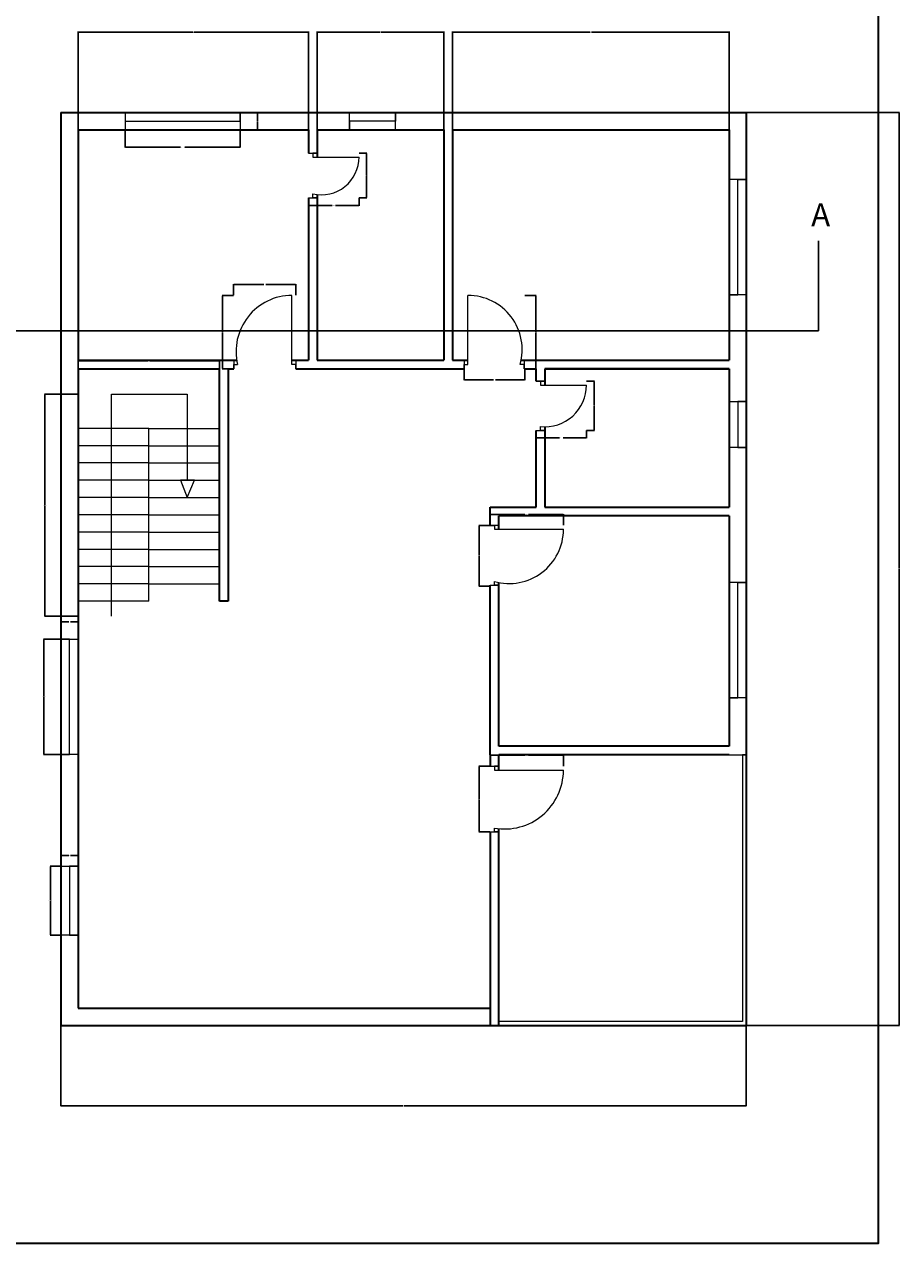
# Model space of a CAD drawing. Units: inches. Extents: x 1912 to 3731, y 1384 to 2459.
# Tile 7 of 8: x 3276 to 3731, y 1384 to 2019. Entities that reach past the tile are written whole.
import ezdxf

# ---------------------------------------------------------------- set-up
doc = ezdxf.new("R2010")
doc.units = ezdxf.units.IN
for name, color, linetype, lineweight in [('A-ANNO-DIMS', 2, 'Continuous', 18), ('A-ANNO-SYMB', 2, 'Continuous', 25), ('A-ANNO-TTLB', 7, 'Continuous', 35), ('A-DOOR', 3, 'Continuous', 20), ('A-FLOR-STRS', 7, 'Continuous', 18), ('A-GLAZ', 4, 'Continuous', 18), ('A-WALL', 7, 'Continuous', 35)]:
    doc.layers.add(name, color=color, linetype=linetype, lineweight=lineweight)
doc.styles.get("Standard").update_dxf_attribs({"font": 'arial.ttf'})
doc.dimstyles.get("Standard").update_dxf_attribs({"dimtxt": 0.18, "dimasz": 0.18, "dimexe": 0.18, "dimexo": 0.0625, "dimgap": 0.09, "dimtad": 0, "dimtih": 1, "dimtoh": 1, "dimdec": 4, "dimzin": 0, "dimdsep": 46, "dimtxsty": 'Standard', "dimcen": 0.09, "dimadec": 0, "dimazin": 0, "dimtfac": 1, "dimtdec": 4, "dimtofl": 0, "dimtmove": 0, "dimatfit": 3, "dimfxl": 1, "dimtolj": 1, "dimtzin": 0, "dimarcsym": 0})

# ---------------------------------------------------------------- blocks, each defined once
blk = doc.blocks.new('STAIR-RETURN-FIRST')
for p, q in [((17.33, 0), (17.33, 115.73)), ((17.33, 115.73), (56.7, 115.73)), ((56.7, 115.73), (56.7, 70.82)), ((36.78, 97.82), (0, 97.82)), ((36.78, 7.82), (36.78, 97.82)), ((36.78, 97.82), (73.56, 97.82)), ((36.78, 88.82), (0, 88.82)), ((36.78, 88.82), (73.56, 88.82)), ((36.78, 79.82), (0, 79.82)), ((36.78, 79.82), (73.56, 79.82)), ((36.78, 70.82), (0, 70.82)), ((36.78, 70.82), (73.56, 70.82)), ((60.6, 70.82), (53.28, 70.82)), ((53.28, 70.82), (56.7, 61.82)), ((56.7, 61.82), (60.6, 70.82)), ((36.78, 61.82), (0, 61.82)), ((36.78, 61.82), (73.56, 61.82)), ((36.78, 52.82), (0, 52.82)), ((36.78, 52.82), (73.56, 52.82)), ((36.78, 43.82), (0, 43.82)), ((36.78, 43.82), (73.56, 43.82)), ((36.78, 34.82), (0, 34.82)), ((36.78, 34.82), (73.56, 34.82)), ((36.78, 25.82), (0, 25.82)), ((36.78, 25.82), (73.56, 25.82)), ((36.78, 16.82), (0, 16.82)), ((36.78, 7.82), (36.78, 16.82)), ((36.78, 16.82), (73.56, 16.82)), ((36.78, 7.82), (0, 7.82))]:
    blk.add_line(p, q)
blk = doc.blocks.new('DOOR-24-FF-ENSUITE')
for p, q in [((0, 23.22), (4.5, 23.22)), ((4.5, 23.22), (2.25, 23.22)), ((2.25, 23.22), (2.25, 21.22)), ((2.25, 21.22), (26.25, 21.22)), ((0, 0), (4.5, 0)), ((2.25, 0), (2.25, 2)), ((4.5, 0), (2.25, 0))]:
    blk.add_line(p, q)
blk.add_arc((6.56, 21.22), 19.69, 257.3694, 0)
blk = doc.blocks.new('DOOR-36-FF-MASTER')
for p, q in [((30.28, 2.25), (30.28, 38.25)), ((0, 4.5), (0, 0)), ((0, 0), (0, 2.25)), ((0, 2.25), (2, 2.25)), ((32.28, 2.25), (30.28, 2.25)), ((32.28, 4.5), (32.28, 0)), ((32.28, 0), (32.28, 2.25))]:
    blk.add_line(p, q)
blk.add_arc((30.28, 9.14), 29.11, 90, 193.70172)
blk = doc.blocks.new('DOOR-36-FF-KIDS')
for p, q in [((2, 2.25), (2, 38.25)), ((0, 4.5), (0, 0)), ((0, 0), (0, 2.25)), ((0, 2.25), (2, 2.25)), ((31.21, 2.25), (29.21, 2.25)), ((31.21, 4.5), (31.21, 0)), ((31.21, 0), (31.21, 2.25))]:
    blk.add_line(p, q)
blk.add_arc((2, 9.97), 28.28, 344.16899, 90)
blk = doc.blocks.new('DOOR-24-FF-BATH')
for p, q in [((0, 25.59), (4.5, 25.59)), ((4.5, 25.59), (0, 25.59)), ((0, 25.59), (2.25, 25.59)), ((2.25, 25.59), (2.25, 23.59)), ((2.25, 23.59), (26.25, 23.59)), ((2.25, 0), (2.25, 2)), ((0, 0), (4.5, 0)), ((4.5, 0), (2.25, 0))]:
    blk.add_line(p, q)
blk.add_arc((4.54, 23.59), 21.71, 263.95392, 0)
blk = doc.blocks.new('DOOR-36-FF-FAMILY')
for p, q in [((4.5, 31.2), (0, 31.2)), ((0, 31.2), (2.25, 31.2)), ((2.25, 31.2), (2.25, 29.2)), ((2.25, 29.2), (38.25, 29.2)), ((2.25, 0), (2.25, 2)), ((0, 0), (4.5, 0)), ((4.5, 0), (2.25, 0))]:
    blk.add_line(p, q)
blk.add_arc((9.98, 29.2), 28.27, 254.13836, 0)
blk = doc.blocks.new('DOOR-36-FF-SUNROOM')
for p, q in [((0, 34.16), (4.5, 34.16)), ((4.5, 34.16), (2.25, 34.16)), ((2.25, 34.16), (2.25, 32.16)), ((2.25, 32.16), (38.25, 32.16)), ((2.25, 0), (2.25, 2)), ((0, 0), (4.5, 0)), ((4.5, 0), (2.25, 0))]:
    blk.add_line(p, q)
blk.add_arc((7.62, 32.16), 30.63, 259.91124, 0)
blk = doc.blocks.new('WIN-PLAN-60-A')
for p, q in [((0, 9), (0, 0)), ((60, 4.5), (60, 9)), ((60, 9), (60, 0)), ((0, 0), (0, 4.5)), ((0, 4.5), (60, 4.5))]:
    blk.add_line(p, q)
blk = doc.blocks.new('WIN-PLAN-60-B')
for p, q in [((0, 60), (9, 60)), ((9, 60), (4.5, 60)), ((4.5, 60), (4.5, 0)), ((9, 0), (0, 0)), ((4.5, 0), (9, 0))]:
    blk.add_line(p, q)
blk = doc.blocks.new('WIN-PLAN-24-A')
for p, q in [((0, 24), (9, 24)), ((9, 24), (4.5, 24)), ((4.5, 24), (4.5, 0)), ((4.5, 0), (0, 0)), ((0, 0), (9, 0))]:
    blk.add_line(p, q)
blk = doc.blocks.new('WIN-PLAN-36')
for p, q in [((4.5, 36), (0, 36)), ((0, 36), (9, 36)), ((4.5, 0), (4.5, 36)), ((9, 0), (0, 0)), ((0, 0), (4.5, 0))]:
    blk.add_line(p, q)
blk = doc.blocks.new('WIN-PLAN-24-B')
for p, q in [((0, 24), (9, 24)), ((9, 24), (4.5, 24)), ((4.5, 24), (4.5, 0)), ((9, 0), (0, 0)), ((4.5, 0), (9, 0))]:
    blk.add_line(p, q)
blk = doc.blocks.new('WIN-PLAN-60-C')
for p, q in [((0, 9), (0, 0)), ((60, 4.5), (60, 9)), ((60, 9), (60, 0)), ((0, 4.5), (60, 4.5))]:
    blk.add_line(p, q)
blk = doc.blocks.new('*D33')
at = {"layer": 'A-ANNO-DIMS', "color": 0, "lineweight": -2, "transparency": 16777216}
for p, q in [((3294.5, 1698.78), (3285.39, 1698.78)), ((3285.57, 1698.6), (3285.57, 1668.97)), ((3285.57, 1638.96), (3285.57, 1668.6)), ((3294.5, 1638.78), (3285.39, 1638.78))]:
    blk.add_line(p, q, dxfattribs=at)
at = {"layer": 'A-ANNO-DIMS', "color": 0, "transparency": 16777216}
for points in [[(3285.54, 1698.6), (3285.6, 1698.6), (3285.57, 1698.78)], [(3285.54, 1638.96), (3285.6, 1638.96), (3285.57, 1638.78)]]:
    blk.add_solid(points, dxfattribs=at)
at = {"layer": 'Defpoints', "color": 0, "transparency": 16777216}
for p in [(3294.57, 1698.78), (3285.57, 1638.78), (3294.57, 1638.78)]:
    blk.add_point(p, dxfattribs=at)
at = {"layer": 'A-ANNO-DIMS', "color": 0, "transparency": 16777216, "insert": (3285.57, 1668.78), "char_height": 0.18, "attachment_point": 5}
blk.add_mtext('\\A1;WINDOW 60 TYP.', dxfattribs=at)
blk = doc.blocks.new('*D34')
at = {"layer": 'A-ANNO-DIMS', "color": 0, "lineweight": -2, "transparency": 16777216}
for p, q in [((3294.57, 1698.85), (3294.57, 1707.96)), ((3294.75, 1707.78), (3298.61, 1707.78)), ((3303.39, 1707.78), (3299.52, 1707.78)), ((3303.57, 1698.85), (3303.57, 1707.96))]:
    blk.add_line(p, q, dxfattribs=at)
at = {"layer": 'A-ANNO-DIMS', "color": 0, "transparency": 16777216}
for points in [[(3294.75, 1707.81), (3294.75, 1707.75), (3294.57, 1707.78)], [(3303.39, 1707.81), (3303.39, 1707.75), (3303.57, 1707.78)]]:
    blk.add_solid(points, dxfattribs=at)
at = {"layer": 'Defpoints', "color": 0, "transparency": 16777216}
for p in [(3294.57, 1707.78), (3294.57, 1698.78), (3303.57, 1698.78)]:
    blk.add_point(p, dxfattribs=at)
at = {"layer": 'A-ANNO-DIMS', "color": 0, "transparency": 16777216, "insert": (3299.07, 1707.78), "char_height": 0.18, "attachment_point": 5}
blk.add_mtext('\\A1;9 TYP.', dxfattribs=at)
blk = doc.blocks.new('*D39')
at = {"layer": 'A-ANNO-DIMS', "color": 0, "lineweight": -2, "transparency": 16777216}
for p, q in [((3294.5, 1580.64), (3288.99, 1580.64)), ((3289.17, 1580.46), (3289.17, 1562.82)), ((3289.17, 1544.82), (3289.17, 1562.45)), ((3294.5, 1544.64), (3288.99, 1544.64))]:
    blk.add_line(p, q, dxfattribs=at)
at = {"layer": 'A-ANNO-DIMS', "color": 0, "transparency": 16777216}
for points in [[(3289.14, 1580.46), (3289.2, 1580.46), (3289.17, 1580.64)], [(3289.14, 1544.82), (3289.2, 1544.82), (3289.17, 1544.64)]]:
    blk.add_solid(points, dxfattribs=at)
at = {"layer": 'Defpoints', "color": 0, "transparency": 16777216}
for p in [(3294.57, 1580.64), (3289.17, 1544.64), (3294.57, 1544.64)]:
    blk.add_point(p, dxfattribs=at)
at = {"layer": 'A-ANNO-DIMS', "color": 0, "transparency": 16777216, "insert": (3289.17, 1562.64), "char_height": 0.18, "attachment_point": 5}
blk.add_mtext('\\A1;WINDOW 36 TYP.', dxfattribs=at)
blk = doc.blocks.new('*D40')
at = {"layer": 'A-ANNO-DIMS', "color": 0, "lineweight": -2, "transparency": 16777216}
for p, q in [((3294.57, 1580.7), (3294.57, 1586.22)), ((3294.75, 1586.04), (3298.61, 1586.04)), ((3303.39, 1586.04), (3299.52, 1586.04)), ((3303.57, 1580.7), (3303.57, 1586.22))]:
    blk.add_line(p, q, dxfattribs=at)
at = {"layer": 'A-ANNO-DIMS', "color": 0, "transparency": 16777216}
for points in [[(3294.75, 1586.07), (3294.75, 1586.01), (3294.57, 1586.04)], [(3303.39, 1586.07), (3303.39, 1586.01), (3303.57, 1586.04)]]:
    blk.add_solid(points, dxfattribs=at)
at = {"layer": 'Defpoints', "color": 0, "transparency": 16777216}
for p in [(3294.57, 1586.04), (3294.57, 1580.64), (3303.57, 1580.64)]:
    blk.add_point(p, dxfattribs=at)
at = {"layer": 'A-ANNO-DIMS', "color": 0, "transparency": 16777216, "insert": (3299.07, 1586.04), "char_height": 0.18, "attachment_point": 5}
blk.add_mtext('\\A1;9 TYP.', dxfattribs=at)
blk = doc.blocks.new('*D41')
at = {"layer": 'A-ANNO-DIMS', "color": 0, "lineweight": -2, "transparency": 16777216}
for p, q in [((3327.96, 1964.06), (3327.96, 1954.95)), ((3387.96, 1964.06), (3387.96, 1954.95)), ((3328.14, 1955.13), (3356.84, 1955.13)), ((3387.78, 1955.13), (3359.08, 1955.13))]:
    blk.add_line(p, q, dxfattribs=at)
at = {"layer": 'A-ANNO-DIMS', "color": 0, "transparency": 16777216}
for points in [[(3328.14, 1955.16), (3328.14, 1955.1), (3327.96, 1955.13)], [(3387.78, 1955.16), (3387.78, 1955.1), (3387.96, 1955.13)]]:
    blk.add_solid(points, dxfattribs=at)
at = {"layer": 'Defpoints', "color": 0, "transparency": 16777216}
for p in [(3327.96, 1964.13), (3387.96, 1964.13), (3387.96, 1955.13)]:
    blk.add_point(p, dxfattribs=at)
at = {"layer": 'A-ANNO-DIMS', "color": 0, "transparency": 16777216, "insert": (3357.96, 1955.13), "char_height": 0.18, "attachment_point": 5}
blk.add_mtext('\\A1;WINDOW 60 TYP.', dxfattribs=at)
blk = doc.blocks.new('*D42')
at = {"layer": 'A-ANNO-DIMS', "color": 0, "lineweight": -2, "transparency": 16777216}
for p, q in [((3388.02, 1973.13), (3397.14, 1973.13)), ((3396.96, 1972.95), (3396.96, 1968.81)), ((3388.02, 1964.13), (3397.14, 1964.13)), ((3396.96, 1964.31), (3396.96, 1968.44))]:
    blk.add_line(p, q, dxfattribs=at)
at = {"layer": 'A-ANNO-DIMS', "color": 0, "transparency": 16777216}
for points in [[(3396.93, 1972.95), (3396.99, 1972.95), (3396.96, 1973.13)], [(3396.93, 1964.31), (3396.99, 1964.31), (3396.96, 1964.13)]]:
    blk.add_solid(points, dxfattribs=at)
at = {"layer": 'Defpoints', "color": 0, "transparency": 16777216}
for p in [(3387.96, 1973.13), (3396.96, 1973.13), (3387.96, 1964.13)]:
    blk.add_point(p, dxfattribs=at)
at = {"layer": 'A-ANNO-DIMS', "color": 0, "transparency": 16777216, "insert": (3396.96, 1968.63), "char_height": 0.18, "attachment_point": 5}
blk.add_mtext('\\A1;9 TYP.', dxfattribs=at)
blk = doc.blocks.new('*D65')
at = {"layer": 'A-ANNO-DIMS', "color": 0, "lineweight": -2, "transparency": 16777216}
for p, q in [((3303.5, 1826.5), (3286.03, 1826.5)), ((3286.21, 1826.32), (3286.21, 1768.82)), ((3286.21, 1710.95), (3286.21, 1768.45)), ((3303.5, 1710.77), (3286.03, 1710.77))]:
    blk.add_line(p, q, dxfattribs=at)
at = {"layer": 'A-ANNO-DIMS', "color": 0, "transparency": 16777216}
for points in [[(3286.18, 1826.32), (3286.24, 1826.32), (3286.21, 1826.5)], [(3286.18, 1710.95), (3286.24, 1710.95), (3286.21, 1710.77)]]:
    blk.add_solid(points, dxfattribs=at)
at = {"layer": 'Defpoints', "color": 0, "transparency": 16777216}
for p in [(3286.21, 1826.5), (3303.57, 1826.5), (3303.57, 1710.77)]:
    blk.add_point(p, dxfattribs=at)
at = {"layer": 'A-ANNO-DIMS', "color": 0, "transparency": 16777216, "insert": (3286.21, 1768.63), "char_height": 0.18, "attachment_point": 5}
blk.add_mtext('\\A1;STAIR 116 TYP.', dxfattribs=at)
blk = doc.blocks.new('*D66')
at = {"layer": 'A-ANNO-DIMS', "color": 0, "lineweight": -2, "transparency": 16777216}
for p, q in [((3303.57, 1826.56), (3303.57, 1844.04)), ((3303.75, 1843.86), (3339.82, 1843.86)), ((3376.94, 1843.86), (3340.87, 1843.86)), ((3377.12, 1826.56), (3377.12, 1844.04))]:
    blk.add_line(p, q, dxfattribs=at)
at = {"layer": 'A-ANNO-DIMS', "color": 0, "transparency": 16777216}
for points in [[(3303.75, 1843.89), (3303.75, 1843.83), (3303.57, 1843.86)], [(3376.94, 1843.89), (3376.94, 1843.83), (3377.12, 1843.86)]]:
    blk.add_solid(points, dxfattribs=at)
at = {"layer": 'Defpoints', "color": 0, "transparency": 16777216}
for p in [(3377.12, 1843.86), (3303.57, 1826.5), (3377.12, 1826.5)]:
    blk.add_point(p, dxfattribs=at)
at = {"layer": 'A-ANNO-DIMS', "color": 0, "transparency": 16777216, "insert": (3340.34, 1843.86), "char_height": 0.18, "attachment_point": 5}
blk.add_mtext('\\A1;74 TYP.', dxfattribs=at)
blk = doc.blocks.new('*D79')
at = {"layer": 'A-ANNO-DIMS', "color": 0, "lineweight": -2, "transparency": 16777216}
for p, q in [((3423.57, 1928.66), (3423.57, 1924.61)), ((3423.75, 1924.79), (3435.76, 1924.79)), ((3449.64, 1924.79), (3437.63, 1924.79)), ((3449.82, 1928.66), (3449.82, 1924.61))]:
    blk.add_line(p, q, dxfattribs=at)
at = {"layer": 'A-ANNO-DIMS', "color": 0, "transparency": 16777216}
for points in [[(3423.75, 1924.82), (3423.75, 1924.76), (3423.57, 1924.79)], [(3449.64, 1924.82), (3449.64, 1924.76), (3449.82, 1924.79)]]:
    blk.add_solid(points, dxfattribs=at)
at = {"layer": 'Defpoints', "color": 0, "transparency": 16777216}
for p in [(3423.57, 1928.72), (3449.82, 1928.72), (3449.82, 1924.79)]:
    blk.add_point(p, dxfattribs=at)
at = {"layer": 'A-ANNO-DIMS', "color": 0, "transparency": 16777216, "insert": (3436.69, 1924.79), "char_height": 0.18, "attachment_point": 5}
blk.add_mtext('\\A1;DOOR 26 TYP.', dxfattribs=at)
blk = doc.blocks.new('*D80')
at = {"layer": 'A-ANNO-DIMS', "color": 0, "lineweight": -2, "transparency": 16777216}
for p, q in [((3449.88, 1951.94), (3453.93, 1951.94)), ((3453.75, 1951.76), (3453.75, 1940.51)), ((3453.75, 1928.9), (3453.75, 1940.15)), ((3449.88, 1928.72), (3453.93, 1928.72))]:
    blk.add_line(p, q, dxfattribs=at)
at = {"layer": 'A-ANNO-DIMS', "color": 0, "transparency": 16777216}
for points in [[(3453.72, 1951.76), (3453.78, 1951.76), (3453.75, 1951.94)], [(3453.72, 1928.9), (3453.78, 1928.9), (3453.75, 1928.72)]]:
    blk.add_solid(points, dxfattribs=at)
at = {"layer": 'Defpoints', "color": 0, "transparency": 16777216}
for p in [(3449.82, 1951.94), (3453.75, 1951.94), (3449.82, 1928.72)]:
    blk.add_point(p, dxfattribs=at)
at = {"layer": 'A-ANNO-DIMS', "color": 0, "transparency": 16777216, "insert": (3453.75, 1940.33), "char_height": 0.18, "attachment_point": 5}
blk.add_mtext('\\A1;23 TYP.', dxfattribs=at)
blk = doc.blocks.new('*D81')
at = {"layer": 'A-ANNO-DIMS', "color": 0, "lineweight": -2, "transparency": 16777216}
for p, q in [((3384.43, 1877.88), (3378.57, 1877.88)), ((3378.75, 1877.7), (3378.75, 1858.93)), ((3378.75, 1839.81), (3378.75, 1858.57)), ((3384.43, 1839.63), (3378.57, 1839.63))]:
    blk.add_line(p, q, dxfattribs=at)
at = {"layer": 'A-ANNO-DIMS', "color": 0, "transparency": 16777216}
for points in [[(3378.72, 1877.7), (3378.78, 1877.7), (3378.75, 1877.88)], [(3378.72, 1839.81), (3378.78, 1839.81), (3378.75, 1839.63)]]:
    blk.add_solid(points, dxfattribs=at)
at = {"layer": 'Defpoints', "color": 0, "transparency": 16777216}
for p in [(3378.75, 1877.88), (3384.49, 1877.88), (3384.49, 1839.63)]:
    blk.add_point(p, dxfattribs=at)
at = {"layer": 'A-ANNO-DIMS', "color": 0, "transparency": 16777216, "insert": (3378.75, 1858.75), "char_height": 0.18, "attachment_point": 5}
blk.add_mtext('\\A1;DOOR 38 TYP.', dxfattribs=at)
blk = doc.blocks.new('*D82')
at = {"layer": 'A-ANNO-DIMS', "color": 0, "lineweight": -2, "transparency": 16777216}
for p, q in [((3384.49, 1877.94), (3384.49, 1883.79)), ((3384.67, 1883.61), (3400.16, 1883.61)), ((3416.7, 1883.61), (3401.21, 1883.61)), ((3416.88, 1877.94), (3416.88, 1883.79))]:
    blk.add_line(p, q, dxfattribs=at)
at = {"layer": 'A-ANNO-DIMS', "color": 0, "transparency": 16777216}
for points in [[(3384.67, 1883.64), (3384.67, 1883.58), (3384.49, 1883.61)], [(3416.7, 1883.64), (3416.7, 1883.58), (3416.88, 1883.61)]]:
    blk.add_solid(points, dxfattribs=at)
at = {"layer": 'Defpoints', "color": 0, "transparency": 16777216}
for p in [(3416.88, 1883.61), (3384.49, 1877.88), (3416.88, 1877.88)]:
    blk.add_point(p, dxfattribs=at)
at = {"layer": 'A-ANNO-DIMS', "color": 0, "transparency": 16777216, "insert": (3400.69, 1883.61), "char_height": 0.18, "attachment_point": 5}
blk.add_mtext('\\A1;32 TYP.', dxfattribs=at)
blk = doc.blocks.new('*D83')
at = {"layer": 'A-ANNO-DIMS', "color": 0, "lineweight": -2, "transparency": 16777216}
for p, q in [((3536.25, 1877.88), (3542.1, 1877.88)), ((3541.92, 1877.7), (3541.92, 1858.93)), ((3541.92, 1839.81), (3541.92, 1858.57)), ((3536.25, 1839.63), (3542.1, 1839.63))]:
    blk.add_line(p, q, dxfattribs=at)
at = {"layer": 'A-ANNO-DIMS', "color": 0, "transparency": 16777216}
for points in [[(3541.89, 1877.7), (3541.95, 1877.7), (3541.92, 1877.88)], [(3541.89, 1839.81), (3541.95, 1839.81), (3541.92, 1839.63)]]:
    blk.add_solid(points, dxfattribs=at)
at = {"layer": 'Defpoints', "color": 0, "transparency": 16777216}
for p in [(3536.19, 1877.88), (3541.92, 1877.88), (3536.19, 1839.63)]:
    blk.add_point(p, dxfattribs=at)
at = {"layer": 'A-ANNO-DIMS', "color": 0, "transparency": 16777216, "insert": (3541.92, 1858.75), "char_height": 0.18, "attachment_point": 5}
blk.add_mtext('\\A1;DOOR 38 TYP.', dxfattribs=at)
blk = doc.blocks.new('*D84')
at = {"layer": 'A-ANNO-DIMS', "color": 0, "lineweight": -2, "transparency": 16777216}
for p, q in [((3504.56, 1839.56), (3504.56, 1833.71)), ((3536.19, 1839.56), (3536.19, 1833.71)), ((3504.74, 1833.89), (3519.84, 1833.89)), ((3536.01, 1833.89), (3520.9, 1833.89))]:
    blk.add_line(p, q, dxfattribs=at)
at = {"layer": 'A-ANNO-DIMS', "color": 0, "transparency": 16777216}
for points in [[(3504.74, 1833.92), (3504.74, 1833.86), (3504.56, 1833.89)], [(3536.01, 1833.92), (3536.01, 1833.86), (3536.19, 1833.89)]]:
    blk.add_solid(points, dxfattribs=at)
at = {"layer": 'Defpoints', "color": 0, "transparency": 16777216}
for p in [(3504.56, 1839.63), (3536.19, 1839.63), (3536.19, 1833.89)]:
    blk.add_point(p, dxfattribs=at)
at = {"layer": 'A-ANNO-DIMS', "color": 0, "transparency": 16777216, "insert": (3520.37, 1833.89), "char_height": 0.18, "attachment_point": 5}
blk.add_mtext('\\A1;32 TYP.', dxfattribs=at)
blk = doc.blocks.new('*D85')
at = {"layer": 'A-ANNO-DIMS', "color": 0, "lineweight": -2, "transparency": 16777216}
for p, q in [((3542.07, 1807.52), (3542.07, 1803.47)), ((3568.32, 1807.52), (3568.32, 1803.47)), ((3542.25, 1803.65), (3554.26, 1803.65)), ((3568.14, 1803.65), (3556.13, 1803.65))]:
    blk.add_line(p, q, dxfattribs=at)
at = {"layer": 'A-ANNO-DIMS', "color": 0, "transparency": 16777216}
for points in [[(3542.25, 1803.68), (3542.25, 1803.62), (3542.07, 1803.65)], [(3568.14, 1803.68), (3568.14, 1803.62), (3568.32, 1803.65)]]:
    blk.add_solid(points, dxfattribs=at)
at = {"layer": 'Defpoints', "color": 0, "transparency": 16777216}
for p in [(3542.07, 1807.58), (3568.32, 1807.58), (3568.32, 1803.65)]:
    blk.add_point(p, dxfattribs=at)
at = {"layer": 'A-ANNO-DIMS', "color": 0, "transparency": 16777216, "insert": (3555.19, 1803.65), "char_height": 0.18, "attachment_point": 5}
blk.add_mtext('\\A1;DOOR 26 TYP.', dxfattribs=at)
blk = doc.blocks.new('*D86')
at = {"layer": 'A-ANNO-DIMS', "color": 0, "lineweight": -2, "transparency": 16777216}
for p, q in [((3568.38, 1833.18), (3572.43, 1833.18)), ((3572.25, 1833), (3572.25, 1820.56)), ((3572.25, 1807.76), (3572.25, 1820.2)), ((3568.38, 1807.58), (3572.43, 1807.58))]:
    blk.add_line(p, q, dxfattribs=at)
at = {"layer": 'A-ANNO-DIMS', "color": 0, "transparency": 16777216}
for points in [[(3572.22, 1833), (3572.28, 1833), (3572.25, 1833.18)], [(3572.22, 1807.76), (3572.28, 1807.76), (3572.25, 1807.58)]]:
    blk.add_solid(points, dxfattribs=at)
at = {"layer": 'Defpoints', "color": 0, "transparency": 16777216}
for p in [(3568.32, 1833.18), (3572.25, 1833.18), (3568.32, 1807.58)]:
    blk.add_point(p, dxfattribs=at)
at = {"layer": 'A-ANNO-DIMS', "color": 0, "transparency": 16777216, "insert": (3572.25, 1820.38), "char_height": 0.18, "attachment_point": 5}
blk.add_mtext('\\A1;26 TYP.', dxfattribs=at)
blk = doc.blocks.new('*D87')
at = {"layer": 'A-ANNO-DIMS', "color": 0, "lineweight": -2, "transparency": 16777216}
for p, q in [((3518.07, 1758.13), (3518.07, 1763.98)), ((3518.25, 1763.8), (3536.26, 1763.8)), ((3556.14, 1763.8), (3538.13, 1763.8)), ((3556.32, 1758.13), (3556.32, 1763.98))]:
    blk.add_line(p, q, dxfattribs=at)
at = {"layer": 'A-ANNO-DIMS', "color": 0, "transparency": 16777216}
for points in [[(3518.25, 1763.83), (3518.25, 1763.77), (3518.07, 1763.8)], [(3556.14, 1763.83), (3556.14, 1763.77), (3556.32, 1763.8)]]:
    blk.add_solid(points, dxfattribs=at)
at = {"layer": 'Defpoints', "color": 0, "transparency": 16777216}
for p in [(3556.32, 1763.8), (3518.07, 1758.07), (3556.32, 1758.07)]:
    blk.add_point(p, dxfattribs=at)
at = {"layer": 'A-ANNO-DIMS', "color": 0, "transparency": 16777216, "insert": (3537.19, 1763.8), "char_height": 0.18, "attachment_point": 5}
blk.add_mtext('\\A1;DOOR 38 TYP.', dxfattribs=at)
blk = doc.blocks.new('*D88')
at = {"layer": 'A-ANNO-DIMS', "color": 0, "lineweight": -2, "transparency": 16777216}
for p, q in [((3518, 1758.07), (3512.15, 1758.07)), ((3512.33, 1757.89), (3512.33, 1742.44)), ((3512.33, 1726.63), (3512.33, 1742.07)), ((3518, 1726.45), (3512.15, 1726.45))]:
    blk.add_line(p, q, dxfattribs=at)
at = {"layer": 'A-ANNO-DIMS', "color": 0, "transparency": 16777216}
for points in [[(3512.3, 1757.89), (3512.36, 1757.89), (3512.33, 1758.07)], [(3512.3, 1726.63), (3512.36, 1726.63), (3512.33, 1726.45)]]:
    blk.add_solid(points, dxfattribs=at)
at = {"layer": 'Defpoints', "color": 0, "transparency": 16777216}
for p in [(3512.33, 1758.07), (3518.07, 1758.07), (3518.07, 1726.45)]:
    blk.add_point(p, dxfattribs=at)
at = {"layer": 'A-ANNO-DIMS', "color": 0, "transparency": 16777216, "insert": (3512.33, 1742.26), "char_height": 0.18, "attachment_point": 5}
blk.add_mtext('\\A1;32 TYP.', dxfattribs=at)
blk = doc.blocks.new('*D89')
at = {"layer": 'A-ANNO-DIMS', "color": 0, "lineweight": -2, "transparency": 16777216}
for p, q in [((3518.07, 1632.64), (3518.07, 1638.49)), ((3518.25, 1638.31), (3536.26, 1638.31)), ((3556.14, 1638.31), (3538.13, 1638.31)), ((3556.32, 1632.64), (3556.32, 1638.49))]:
    blk.add_line(p, q, dxfattribs=at)
at = {"layer": 'A-ANNO-DIMS', "color": 0, "transparency": 16777216}
for points in [[(3518.25, 1638.34), (3518.25, 1638.28), (3518.07, 1638.31)], [(3556.14, 1638.34), (3556.14, 1638.28), (3556.32, 1638.31)]]:
    blk.add_solid(points, dxfattribs=at)
at = {"layer": 'Defpoints', "color": 0, "transparency": 16777216}
for p in [(3518.07, 1632.58), (3556.32, 1638.31), (3556.32, 1632.58)]:
    blk.add_point(p, dxfattribs=at)
at = {"layer": 'A-ANNO-DIMS', "color": 0, "transparency": 16777216, "insert": (3537.19, 1638.31), "char_height": 0.18, "attachment_point": 5}
blk.add_mtext('\\A1;DOOR 38 TYP.', dxfattribs=at)
blk = doc.blocks.new('*D90')
at = {"layer": 'A-ANNO-DIMS', "color": 0, "lineweight": -2, "transparency": 16777216}
for p, q in [((3518, 1632.58), (3512.15, 1632.58)), ((3512.33, 1632.4), (3512.33, 1615.68)), ((3512.33, 1598.6), (3512.33, 1615.31)), ((3518, 1598.42), (3512.15, 1598.42))]:
    blk.add_line(p, q, dxfattribs=at)
at = {"layer": 'A-ANNO-DIMS', "color": 0, "transparency": 16777216}
for points in [[(3512.3, 1632.4), (3512.36, 1632.4), (3512.33, 1632.58)], [(3512.3, 1598.6), (3512.36, 1598.6), (3512.33, 1598.42)]]:
    blk.add_solid(points, dxfattribs=at)
at = {"layer": 'Defpoints', "color": 0, "transparency": 16777216}
for p in [(3512.33, 1632.58), (3518.07, 1632.58), (3518.07, 1598.42)]:
    blk.add_point(p, dxfattribs=at)
at = {"layer": 'A-ANNO-DIMS', "color": 0, "transparency": 16777216, "insert": (3512.33, 1615.5), "char_height": 0.18, "attachment_point": 5}
blk.add_mtext('\\A1;34 TYP.', dxfattribs=at)
blk = doc.blocks.new('*D106')
at = {"layer": 'A-ANNO-DIMS', "color": 0, "lineweight": -2, "transparency": 16777216}
for p, q in [((3294.57, 1497.56), (3294.57, 1455.5)), ((3651.57, 1497.56), (3651.57, 1455.5)), ((3294.75, 1455.68), (3472.78, 1455.68)), ((3651.39, 1455.68), (3473.35, 1455.68))]:
    blk.add_line(p, q, dxfattribs=at)
at = {"layer": 'A-ANNO-DIMS', "color": 0, "transparency": 16777216}
for points in [[(3294.75, 1455.71), (3294.75, 1455.65), (3294.57, 1455.68)], [(3651.39, 1455.71), (3651.39, 1455.65), (3651.57, 1455.68)]]:
    blk.add_solid(points, dxfattribs=at)
at = {"layer": 'Defpoints', "color": 0, "transparency": 16777216}
for p in [(3294.57, 1497.63), (3651.57, 1497.63), (3651.57, 1455.68)]:
    blk.add_point(p, dxfattribs=at)
at = {"layer": 'A-ANNO-DIMS', "color": 0, "transparency": 16777216, "insert": (3473.07, 1455.68), "char_height": 0.18, "attachment_point": 5}
blk.add_mtext('\\A1;357', dxfattribs=at)
blk = doc.blocks.new('*D107')
at = {"layer": 'A-ANNO-DIMS', "color": 0, "lineweight": -2, "transparency": 16777216}
for p, q in [((3651.63, 1973.13), (3731.29, 1973.13)), ((3731.11, 1972.95), (3731.11, 1735.56)), ((3731.11, 1497.81), (3731.11, 1735.19)), ((3651.63, 1497.63), (3731.29, 1497.63))]:
    blk.add_line(p, q, dxfattribs=at)
at = {"layer": 'A-ANNO-DIMS', "color": 0, "transparency": 16777216}
for points in [[(3731.08, 1972.95), (3731.14, 1972.95), (3731.11, 1973.13)], [(3731.08, 1497.81), (3731.14, 1497.81), (3731.11, 1497.63)]]:
    blk.add_solid(points, dxfattribs=at)
at = {"layer": 'Defpoints', "color": 0, "transparency": 16777216}
for p in [(3651.57, 1973.13), (3731.11, 1973.13), (3651.57, 1497.63)]:
    blk.add_point(p, dxfattribs=at)
at = {"layer": 'A-ANNO-DIMS', "color": 0, "transparency": 16777216, "insert": (3731.11, 1735.38), "char_height": 0.18, "attachment_point": 5}
blk.add_mtext('\\A1;475.5', dxfattribs=at)
blk = doc.blocks.new('*D112')
at = {"layer": 'A-ANNO-DIMS', "color": 0, "lineweight": -2, "transparency": 16777216}
for p, q in [((3303.57, 1964.19), (3303.57, 2015.26)), ((3303.75, 2015.08), (3363.29, 2015.08)), ((3423.39, 2015.08), (3363.85, 2015.08)), ((3423.57, 1964.19), (3423.57, 2015.26))]:
    blk.add_line(p, q, dxfattribs=at)
at = {"layer": 'A-ANNO-DIMS', "color": 0, "transparency": 16777216}
for points in [[(3303.75, 2015.11), (3303.75, 2015.05), (3303.57, 2015.08)], [(3423.39, 2015.11), (3423.39, 2015.05), (3423.57, 2015.08)]]:
    blk.add_solid(points, dxfattribs=at)
at = {"layer": 'Defpoints', "color": 0, "transparency": 16777216}
for p in [(3423.57, 2015.08), (3303.57, 1964.13), (3423.57, 1964.13)]:
    blk.add_point(p, dxfattribs=at)
at = {"layer": 'A-ANNO-DIMS', "color": 0, "transparency": 16777216, "insert": (3363.57, 2015.08), "char_height": 0.18, "attachment_point": 5}
blk.add_mtext('\\A1;120', dxfattribs=at)
blk = doc.blocks.new('*D113')
at = {"layer": 'A-ANNO-DIMS', "color": 0, "lineweight": -2, "transparency": 16777216}
for p, q in [((3428.07, 1964.19), (3428.07, 2015.26)), ((3428.25, 2015.08), (3460.85, 2015.08)), ((3493.89, 2015.08), (3461.29, 2015.08)), ((3494.07, 1964.19), (3494.07, 2015.26))]:
    blk.add_line(p, q, dxfattribs=at)
at = {"layer": 'A-ANNO-DIMS', "color": 0, "transparency": 16777216}
for points in [[(3428.25, 2015.11), (3428.25, 2015.05), (3428.07, 2015.08)], [(3493.89, 2015.11), (3493.89, 2015.05), (3494.07, 2015.08)]]:
    blk.add_solid(points, dxfattribs=at)
at = {"layer": 'Defpoints', "color": 0, "transparency": 16777216}
for p in [(3494.07, 2015.08), (3428.07, 1964.13), (3494.07, 1964.13)]:
    blk.add_point(p, dxfattribs=at)
at = {"layer": 'A-ANNO-DIMS', "color": 0, "transparency": 16777216, "insert": (3461.07, 2015.08), "char_height": 0.18, "attachment_point": 5}
blk.add_mtext('\\A1;66', dxfattribs=at)
blk = doc.blocks.new('*D114')
at = {"layer": 'A-ANNO-DIMS', "color": 0, "lineweight": -2, "transparency": 16777216}
for p, q in [((3498.57, 1964.19), (3498.57, 2015.26)), ((3498.75, 2015.08), (3570.29, 2015.08)), ((3642.39, 2015.08), (3570.85, 2015.08)), ((3642.57, 1964.19), (3642.57, 2015.26))]:
    blk.add_line(p, q, dxfattribs=at)
at = {"layer": 'A-ANNO-DIMS', "color": 0, "transparency": 16777216}
for points in [[(3498.75, 2015.11), (3498.75, 2015.05), (3498.57, 2015.08)], [(3642.39, 2015.11), (3642.39, 2015.05), (3642.57, 2015.08)]]:
    blk.add_solid(points, dxfattribs=at)
at = {"layer": 'Defpoints', "color": 0, "transparency": 16777216}
for p in [(3642.57, 2015.08), (3498.57, 1964.13), (3642.57, 1964.13)]:
    blk.add_point(p, dxfattribs=at)
at = {"layer": 'A-ANNO-DIMS', "color": 0, "transparency": 16777216, "insert": (3570.57, 2015.08), "char_height": 0.18, "attachment_point": 5}
blk.add_mtext('\\A1;144', dxfattribs=at)

msp = doc.modelspace()

# ---------------------------------------------------------------- linework, layer by layer
at = {"layer": 'A-ANNO-SYMB'}
for p, q in [((3689.1639, 1859.4655), (3689.1639, 1906.3694)), ((2865.8394, 1859.4655), (3689.1639, 1859.4655))]:
    msp.add_line(p, q, dxfattribs=at)
at = {"layer": 'A-ANNO-TTLB'}
msp.add_lwpolyline([(1912.2029, 2458.5537), (3720.218, 2458.5537), (3720.218, 1383.9599), (1912.2029, 1383.9599)], close=True, dxfattribs=at)
at = {"layer": 'A-GLAZ'}
for p, q in [((3642.5659, 1638.6258), (3651.5659, 1638.6258)), ((3651.5659, 1638.6258), (3649.5659, 1638.6258)), ((3649.5659, 1638.6258), (3649.5659, 1499.6258)), ((3649.5659, 1499.6258), (3522.5659, 1499.6258))]:
    msp.add_line(p, q, dxfattribs=at)
at = {"layer": 'A-WALL'}
for p, q in [((3294.5659, 1973.1258), (3651.5659, 1973.1258)), ((3294.5659, 1973.1258), (3294.5659, 1497.6258)), ((3651.5659, 1973.1258), (3651.5659, 1497.6258)), ((3303.5659, 1964.1258), (3423.5659, 1964.1258)), ((3303.5659, 1964.1258), (3303.5659, 1844.1258)), ((3423.5659, 1964.1258), (3423.5659, 1951.9406)), ((3428.0659, 1964.1258), (3494.0659, 1964.1258)), ((3428.0659, 1964.1258), (3428.0659, 1949.9406)), ((3494.0659, 1964.1258), (3494.0659, 1844.1258)), ((3498.5659, 1964.1258), (3642.5659, 1964.1258)), ((3498.5659, 1964.1258), (3498.5659, 1844.1258)), ((3642.5659, 1964.1258), (3642.5659, 1844.1258)), ((3423.5659, 1928.7235), (3423.5659, 1844.1258)), ((3428.0659, 1930.3545), (3428.0659, 1844.1258)), ((3303.5659, 1844.1258), (3386.1492, 1844.1258)), ((3414.882, 1844.1258), (3423.5659, 1844.1258)), ((3428.0659, 1844.1258), (3494.0659, 1844.1258)), ((3498.5659, 1844.1258), (3506.5559, 1844.1258)), ((3534.3068, 1844.1258), (3642.5659, 1844.1258)), ((3303.5659, 1839.6258), (3377.1233, 1839.6258)), ((3303.5659, 1839.6258), (3303.5659, 1506.6258)), ((3377.1233, 1718.5838), (3377.1233, 1839.6258)), ((3381.6233, 1839.6258), (3384.6045, 1839.6258)), ((3381.6233, 1839.6258), (3381.6233, 1718.5838)), ((3416.882, 1839.6258), (3504.5559, 1839.6258)), ((3535.7671, 1839.6258), (3542.0659, 1839.6258)), ((3542.0659, 1833.1769), (3542.0659, 1839.6258)), ((3546.5659, 1839.6258), (3642.5659, 1839.6258)), ((3642.5659, 1839.6258), (3546.5659, 1839.6258)), ((3546.5659, 1839.6258), (3546.5659, 1831.1769)), ((3642.5659, 1839.6258), (3642.5659, 1767.6258)), ((3542.0659, 1767.6258), (3542.0659, 1807.5847)), ((3546.5659, 1809.4639), (3546.5659, 1767.6258)), ((3518.0659, 1758.0661), (3518.0659, 1767.6258)), ((3518.0659, 1767.6258), (3542.0659, 1767.6258)), ((3546.5659, 1767.6258), (3642.5659, 1767.6258)), ((3522.5659, 1756.0661), (3522.5659, 1763.1258)), ((3542.0659, 1763.1258), (3522.5659, 1763.1258)), ((3546.5659, 1763.1258), (3542.0659, 1763.1258)), ((3642.5659, 1763.1258), (3546.5659, 1763.1258)), ((3642.5659, 1763.1258), (3642.5659, 1643.1258)), ((3522.5659, 1643.1258), (3522.5659, 1728.3291)), ((3518.0659, 1638.6258), (3518.0659, 1726.8699)), ((3381.6233, 1718.5838), (3377.1233, 1718.5838)), ((3518.0659, 1638.6258), (3518.0659, 1632.5769)), ((3642.5659, 1643.1258), (3522.5659, 1643.1258)), ((3546.5659, 1638.6258), (3522.5659, 1638.6258)), ((3522.5659, 1630.5769), (3522.5659, 1638.6258)), ((3642.5659, 1643.1258), (3546.5659, 1643.1258)), ((3642.5659, 1638.6258), (3546.5659, 1638.6258)), ((3518.0659, 1598.4168), (3518.0659, 1497.6258)), ((3522.5659, 1497.6258), (3522.5659, 1600.1021)), ((3303.5659, 1506.6258), (3518.0659, 1506.6258)), ((3294.5659, 1497.6258), (3651.5659, 1497.6258)), ((3518.0659, 1497.6258), (3522.5659, 1497.6258))]:
    msp.add_line(p, q, dxfattribs=at)

# ---------------------------------------------------------------- block references
at = {"layer": 'A-DOOR'}
for name, p in [('DOOR-24-FF-ENSUITE', (3423.5658, 1928.723)), ('DOOR-36-FF-MASTER', (3384.6048, 1839.626)), ('DOOR-36-FF-KIDS', (3504.5558, 1839.626)), ('DOOR-24-FF-BATH', (3542.0658, 1807.585)), ('DOOR-36-FF-FAMILY', (3518.0658, 1726.87)), ('DOOR-36-FF-SUNROOM', (3518.0658, 1598.417))]:
    msp.add_blockref(name, p, dxfattribs=at)
at = {"layer": 'A-FLOR-STRS'}
msp.add_blockref('STAIR-RETURN-FIRST', (3303.5658, 1710.768), dxfattribs=at)
at = {"layer": 'A-GLAZ'}
for name, p in [('WIN-PLAN-60-C', (3327.9568, 1964.126)), ('WIN-PLAN-24-B', (3642.5658, 1798.63))]:
    msp.add_blockref(name, p, dxfattribs=at)
at = {"layer": 'A-GLAZ', "extrusion": (0, 0, -1), "zscale": -1, "rotation": 90}
for name, p in [('WIN-PLAN-24-A', (-3444.9039, 1964.126)), ('WIN-PLAN-60-A', (-3642.5661, 1878.2056)), ('WIN-PLAN-60-A', (-3642.5661, 1668.3249))]:
    msp.add_blockref(name, p, dxfattribs=at)
at = {"layer": 'A-GLAZ', "rotation": 180}
for name, p in [('WIN-PLAN-60-B', (3303.5657, 1698.7837)), ('WIN-PLAN-36', (3303.5657, 1580.6377))]:
    msp.add_blockref(name, p, dxfattribs=at)

# ---------------------------------------------------------------- texts
at = {"layer": 'A-ANNO-SYMB', "insert": (3685.3296, 1925.8478), "char_height": 12, "attachment_point": 1}
msp.add_mtext_dynamic_manual_height_columns('A', width=24.256269, gutter_width=12.5, heights=[0], dxfattribs=at)

# ---------------------------------------------------------------- dimensions: what is measured, and where the dimension line sits
at = {"layer": 'A-ANNO-DIMS'}
for base, p1, p2, picture, middle in [((3423.5659, 2015.0758), (3303.5659, 1964.1258), (3423.5659, 1964.1258), '*D112', (3363.5659, 2015.0758)), ((3494.0659, 2015.0758), (3428.0659, 1964.1258), (3494.0659, 1964.1258), '*D113', (3461.0659, 2015.0758)), ((3642.5659, 2015.0758), (3498.5659, 1964.1258), (3642.5659, 1964.1258), '*D114', (3570.5659, 2015.0758)), ((3651.5659, 1455.6758), (3294.5659, 1497.6258), (3651.5659, 1497.6258), '*D106', (3473.0659, 1455.6758))]:
    dim = msp.add_linear_dim(base=base, p1=p1, p2=p2, dimstyle='Standard', override={"dimdec": 0, "dimlfac": 1, "dimrnd": 0, "dimzin": 0, "dimdsep": 46, "dimlunit": 2}, dxfattribs=at)
    dim.commit()
    dim.dimension.update_dxf_attribs({"geometry": picture, "text_midpoint": middle})
for base, p1, p2, angle, text, picture, middle in [((3396.9573, 1973.1258), (3387.9573, 1964.1258), (3387.9573, 1973.1258), 90, '<> TYP.', '*D42', (3396.9573, 1968.6258)), ((3453.7534, 1951.9406), (3449.8159, 1928.7235), (3449.8159, 1951.9406), 90, '<> TYP.', '*D80', (3453.7534, 1940.332)), ((3378.7511, 1877.8758), (3384.4886, 1839.6258), (3384.4886, 1877.8758), 90, 'DOOR <> TYP.', '*D81', (3378.7511, 1858.7508)), ((3541.9231, 1877.8758), (3536.1856, 1839.6258), (3536.1856, 1877.8758), 90, 'DOOR <> TYP.', '*D83', (3541.9231, 1858.7508)), ((3572.2534, 1833.1769), (3568.3159, 1807.5847), (3568.3159, 1833.1769), 90, '<> TYP.', '*D86', (3572.2534, 1820.3808)), ((3286.2057, 1826.502), (3303.5659, 1710.7677), (3303.5659, 1826.502), 90, 'STAIR <> TYP.', '*D65', (3286.2057, 1768.6348)), ((3512.3284, 1758.0661), (3518.0659, 1726.4471), (3518.0659, 1758.0661), 90, '<> TYP.', '*D88', (3512.3284, 1742.2566)), ((3294.5659, 1707.7838), (3303.5659, 1698.7838), (3294.5659, 1698.7838), 180, '<> TYP.', '*D34', (3299.0659, 1707.7838)), ((3285.5659, 1638.7838), (3294.5659, 1698.7838), (3294.5659, 1638.7838), 270, 'WINDOW <> TYP.', '*D33', (3285.5659, 1668.7838)), ((3512.3284, 1632.5769), (3518.0659, 1598.4168), (3518.0659, 1632.5769), 90, '<> TYP.', '*D90', (3512.3284, 1615.4969)), ((3294.5659, 1586.0379), (3303.5659, 1580.6379), (3294.5659, 1580.6379), 180, '<> TYP.', '*D40', (3299.0659, 1586.0379)), ((3289.1659, 1544.6379), (3294.5659, 1580.6379), (3294.5659, 1544.6379), 270, 'WINDOW <> TYP.', '*D39', (3289.1659, 1562.6379))]:
    dim = msp.add_linear_dim(base=base, p1=p1, p2=p2, angle=angle, text=text, dimstyle='Standard', override={"dimdec": 0, "dimlfac": 1, "dimrnd": 0, "dimzin": 0, "dimdsep": 46, "dimlunit": 2}, dxfattribs=at)
    dim.commit()
    dim.dimension.update_dxf_attribs({"geometry": picture, "text_midpoint": middle})
dim = msp.add_linear_dim(base=(3731.1139, 1973.1258), p1=(3651.5659, 1497.6258), p2=(3651.5659, 1973.1258), angle=90, dimstyle='Standard', override={"dimdec": 1, "dimlfac": 1, "dimrnd": 0, "dimzin": 0, "dimdsep": 46, "dimlunit": 2}, dxfattribs=at)
dim.commit()
dim.dimension.update_dxf_attribs({"geometry": '*D107', "text_midpoint": (3731.1139, 1735.3758)})
for base, p1, p2, text, picture, middle in [((3387.9573, 1955.1258), (3327.9573, 1964.1258), (3387.9573, 1964.1258), 'WINDOW <> TYP.', '*D41', (3357.9573, 1955.1258)), ((3449.8159, 1924.786), (3423.5659, 1928.7235), (3449.8159, 1928.7235), 'DOOR <> TYP.', '*D79', (3436.6909, 1924.786)), ((3416.882, 1883.6133), (3384.4886, 1877.8758), (3416.882, 1877.8758), '<> TYP.', '*D82', (3400.6853, 1883.6133)), ((3377.1233, 1843.8621), (3303.5659, 1826.502), (3377.1233, 1826.502), '<> TYP.', '*D66', (3340.3446, 1843.8621)), ((3536.1856, 1833.8883), (3504.5559, 1839.6258), (3536.1856, 1839.6258), '<> TYP.', '*D84', (3520.3707, 1833.8883)), ((3568.3159, 1803.6472), (3542.0659, 1807.5847), (3568.3159, 1807.5847), 'DOOR <> TYP.', '*D85', (3555.1909, 1803.6472)), ((3556.3159, 1763.8036), (3518.0659, 1758.0661), (3556.3159, 1758.0661), 'DOOR <> TYP.', '*D87', (3537.1909, 1763.8036)), ((3556.3159, 1638.3144), (3518.0659, 1632.5769), (3556.3159, 1632.5769), 'DOOR <> TYP.', '*D89', (3537.1909, 1638.3144))]:
    dim = msp.add_linear_dim(base=base, p1=p1, p2=p2, text=text, dimstyle='Standard', override={"dimdec": 0, "dimlfac": 1, "dimrnd": 0, "dimzin": 0, "dimdsep": 46, "dimlunit": 2}, dxfattribs=at)
    dim.commit()
    dim.dimension.update_dxf_attribs({"geometry": picture, "text_midpoint": middle})

doc.saveas('drawing.dxf')
